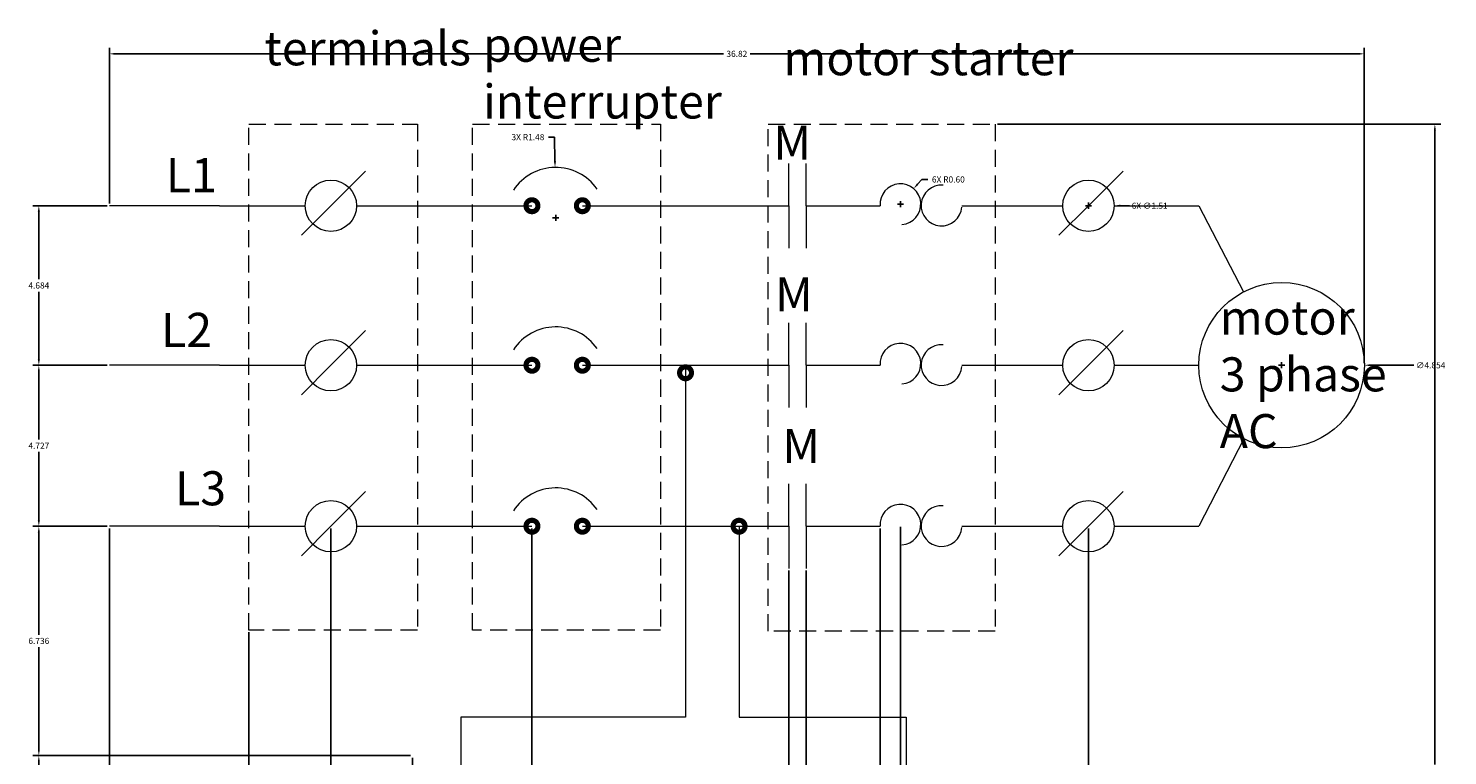
# Model space of a CAD drawing. Units: millimetres. Extents: x 39.4 to 81, y 9.5 to 52.5.
# Tile 2 of 2: x 39.4 to 81, y 31.2 to 52.5. Entities that reach past the tile are written whole.
import ezdxf

# ---------------------------------------------------------------- set-up
doc = ezdxf.new("R2010")
doc.units = ezdxf.units.MM
doc.header["$MEASUREMENT"] = 0
doc.linetypes.add('HIDDENX2', pattern=[0.75, 0.5, -0.25])
for name, color, linetype, lineweight in [('A-ANNO-DIMS', 2, 'Continuous', 18), ('E-ANNO-TEXT', 7, 'Continuous', 13), ('E-DIAG-CONN', 7, 'Continuous', 18), ('E-DIAG-PROT', 7, 'Continuous', 18), ('E-EQPM-BNDY', 8, 'HIDDENX2', 13), ('E-POWR-EQPM', 7, 'Continuous', 20), ('E-POWR-WIRE', 7, 'Continuous', 18)]:
    doc.layers.add(name, color=color, linetype=linetype, lineweight=lineweight)
doc.styles.get("Standard").update_dxf_attribs({"font": 'arial.ttf'})
doc.dimstyles.get("Standard").update_dxf_attribs({"dimtxt": 0.18, "dimasz": 0.18, "dimexe": 0.18, "dimexo": 0.0625, "dimgap": 0.09, "dimtad": 0, "dimtih": 1, "dimtoh": 1, "dimdec": 4, "dimzin": 0, "dimdsep": 46, "dimtxsty": 'Standard', "dimcen": 0.09, "dimadec": 0, "dimazin": 0, "dimtfac": 1, "dimtdec": 4, "dimtofl": 0, "dimtmove": 0, "dimatfit": 3, "dimfxl": 1, "dimtolj": 1, "dimtzin": 0, "dimarcsym": 0})

# ---------------------------------------------------------------- blocks, each defined once
blk = doc.blocks.new('SCREW-TERMINAL')
for q in [(1.883, 1.883), (0, 0)]:
    blk.add_line((0.865, 0.865), q)
blk.add_circle((0.865, 0.865), 0.753)
blk = doc.blocks.new('INTERRUPTER-POLE')
at = {"const_width": 0.15}
for points in [[(0.367, 0.175, 1), (0.717, 0.175, 1)], [(1.846, 0.175, 1), (2.196, 0.175, 1)]]:
    blk.add_lwpolyline(points, format="xyb", close=True, dxfattribs=at)
blk.add_arc((1.239, -0.182), 1.482, 34.8147, 146.7068)
blk = doc.blocks.new('CONTACTOR-NO-POLE')
for p, q in [((0, 1.242), (0, 2.485)), ((0.513, 1.242), (0.513, 2.485)), ((0, 1.242), (0, 0)), ((0.513, 1.242), (0.513, 0))]:
    blk.add_line(p, q)
blk = doc.blocks.new('OVERLOAD-HEATER')
for centre, start, end in [((0.597, 0.638), 274.3585, 184.3585), ((1.802, 0.598), 85.6415, 355.6415)]:
    blk.add_arc(centre, 0.598, start, end)
blk = doc.blocks.new('WIRE-JUNCTION')
at = {"const_width": 0.15}
blk.add_lwpolyline([(0, 0.175, 1), (0.35, 0.175, 1)], format="xyb", close=True, dxfattribs=at)
blk = doc.blocks.new('*D6')
at = {"layer": 'A-ANNO-DIMS', "color": 0, "lineweight": -2, "transparency": 16777216}
for p, q in [((41.706, 47.307), (39.52, 47.307)), ((39.7, 47.127), (39.7, 45.147)), ((39.7, 42.803), (39.7, 44.783)), ((41.706, 42.623), (39.52, 42.623))]:
    blk.add_line(p, q, dxfattribs=at)
at = {"layer": 'A-ANNO-DIMS', "color": 0, "transparency": 16777216}
for points in [[(39.67, 47.127), (39.73, 47.127), (39.7, 47.307)], [(39.67, 42.803), (39.73, 42.803), (39.7, 42.623)]]:
    blk.add_solid(points, dxfattribs=at)
at = {"layer": 'Defpoints', "color": 0, "transparency": 16777216}
for p in [(41.769, 47.307), (39.7, 42.623), (41.769, 42.623)]:
    blk.add_point(p, dxfattribs=at)
at = {"layer": 'A-ANNO-DIMS', "color": 0, "transparency": 16777216, "insert": (39.7, 44.965), "char_height": 0.18, "attachment_point": 5}
blk.add_mtext('\\A1;4.684', dxfattribs=at)
blk = doc.blocks.new('*D7')
at = {"layer": 'A-ANNO-DIMS', "color": 0, "lineweight": -2, "transparency": 16777216}
for p, q in [((41.706, 42.623), (39.52, 42.623)), ((39.7, 42.443), (39.7, 40.44)), ((39.7, 38.076), (39.7, 40.079)), ((41.706, 37.896), (39.52, 37.896))]:
    blk.add_line(p, q, dxfattribs=at)
at = {"layer": 'A-ANNO-DIMS', "color": 0, "transparency": 16777216}
for points in [[(39.67, 42.443), (39.73, 42.443), (39.7, 42.623)], [(39.67, 38.076), (39.73, 38.076), (39.7, 37.896)]]:
    blk.add_solid(points, dxfattribs=at)
at = {"layer": 'Defpoints', "color": 0, "transparency": 16777216}
for p in [(41.769, 42.623), (39.7, 37.896), (41.769, 37.896)]:
    blk.add_point(p, dxfattribs=at)
at = {"layer": 'A-ANNO-DIMS', "color": 0, "transparency": 16777216, "insert": (39.7, 40.26), "char_height": 0.18, "attachment_point": 5}
blk.add_mtext('\\A1;4.727', dxfattribs=at)
blk = doc.blocks.new('*D8')
at = {"layer": 'A-ANNO-DIMS', "color": 0, "lineweight": -2, "transparency": 16777216}
for p, q in [((41.706, 37.896), (39.52, 37.896)), ((39.7, 37.716), (39.7, 34.71)), ((39.7, 31.339), (39.7, 34.346)), ((50.604, 31.159), (39.52, 31.159))]:
    blk.add_line(p, q, dxfattribs=at)
at = {"layer": 'A-ANNO-DIMS', "color": 0, "transparency": 16777216}
for points in [[(39.67, 37.716), (39.73, 37.716), (39.7, 37.896)], [(39.67, 31.339), (39.73, 31.339), (39.7, 31.159)]]:
    blk.add_solid(points, dxfattribs=at)
at = {"layer": 'Defpoints', "color": 0, "transparency": 16777216}
for p in [(41.769, 37.896), (39.7, 31.159), (50.667, 31.159)]:
    blk.add_point(p, dxfattribs=at)
at = {"layer": 'A-ANNO-DIMS', "color": 0, "transparency": 16777216, "insert": (39.7, 34.528), "char_height": 0.18, "attachment_point": 5}
blk.add_mtext('\\A1;6.736', dxfattribs=at)
blk = doc.blocks.new('*D9')
at = {"layer": 'A-ANNO-DIMS', "color": 0, "lineweight": -2, "transparency": 16777216}
for p, q in [((50.604, 31.159), (39.52, 31.159)), ((39.7, 30.979), (39.7, 28.521)), ((39.7, 25.698), (39.7, 28.157)), ((49.021, 25.518), (39.52, 25.518))]:
    blk.add_line(p, q, dxfattribs=at)
at = {"layer": 'A-ANNO-DIMS', "color": 0, "transparency": 16777216}
for points in [[(39.67, 30.979), (39.73, 30.979), (39.7, 31.159)], [(39.67, 25.698), (39.73, 25.698), (39.7, 25.518)]]:
    blk.add_solid(points, dxfattribs=at)
at = {"layer": 'Defpoints', "color": 0, "transparency": 16777216}
for p in [(50.667, 31.159), (39.7, 25.518), (49.084, 25.518)]:
    blk.add_point(p, dxfattribs=at)
at = {"layer": 'A-ANNO-DIMS', "color": 0, "transparency": 16777216, "insert": (39.7, 28.339), "char_height": 0.18, "attachment_point": 5}
blk.add_mtext('\\A1;5.641', dxfattribs=at)
blk = doc.blocks.new('*D12')
at = {"layer": 'A-ANNO-DIMS', "color": 0, "lineweight": -2, "transparency": 16777216}
for p, q in [((41.769, 37.833), (41.769, 9.486)), ((48.27, 37.833), (48.27, 9.486)), ((41.949, 9.666), (44.643, 9.666)), ((48.09, 9.666), (45.396, 9.666))]:
    blk.add_line(p, q, dxfattribs=at)
at = {"layer": 'A-ANNO-DIMS', "color": 0, "transparency": 16777216}
for points in [[(41.949, 9.696), (41.949, 9.636), (41.769, 9.666)], [(48.09, 9.696), (48.09, 9.636), (48.27, 9.666)]]:
    blk.add_solid(points, dxfattribs=at)
at = {"layer": 'Defpoints', "color": 0, "transparency": 16777216}
for p in [(41.769, 37.896), (48.27, 37.896), (48.27, 9.666)]:
    blk.add_point(p, dxfattribs=at)
at = {"layer": 'A-ANNO-DIMS', "color": 0, "transparency": 16777216, "insert": (45.02, 9.666), "char_height": 0.18, "attachment_point": 5}
blk.add_mtext('\\A1;6.501', dxfattribs=at)
blk = doc.blocks.new('*D13')
at = {"layer": 'A-ANNO-DIMS', "color": 0, "lineweight": -2, "transparency": 16777216}
for p, q in [((48.27, 37.833), (48.27, 9.486)), ((54.169, 37.833), (54.169, 9.486)), ((48.45, 9.666), (50.826, 9.666)), ((53.989, 9.666), (51.614, 9.666))]:
    blk.add_line(p, q, dxfattribs=at)
at = {"layer": 'A-ANNO-DIMS', "color": 0, "transparency": 16777216}
for points in [[(48.45, 9.696), (48.45, 9.636), (48.27, 9.666)], [(53.989, 9.696), (53.989, 9.636), (54.169, 9.666)]]:
    blk.add_solid(points, dxfattribs=at)
at = {"layer": 'Defpoints', "color": 0, "transparency": 16777216}
for p in [(48.27, 37.896), (54.169, 37.896), (54.169, 9.666)]:
    blk.add_point(p, dxfattribs=at)
at = {"layer": 'A-ANNO-DIMS', "color": 0, "transparency": 16777216, "insert": (51.22, 9.666), "char_height": 0.18, "attachment_point": 5}
blk.add_mtext('\\A1;5.899', dxfattribs=at)
blk = doc.blocks.new('*D14')
at = {"layer": 'A-ANNO-DIMS', "color": 0, "lineweight": -2, "transparency": 16777216}
for p, q in [((54.169, 37.833), (54.169, 9.486)), ((61.702, 36.591), (61.702, 9.486)), ((54.349, 9.666), (57.543, 9.666)), ((61.522, 9.666), (58.329, 9.666))]:
    blk.add_line(p, q, dxfattribs=at)
at = {"layer": 'A-ANNO-DIMS', "color": 0, "transparency": 16777216}
for points in [[(54.349, 9.696), (54.349, 9.636), (54.169, 9.666)], [(61.522, 9.696), (61.522, 9.636), (61.702, 9.666)]]:
    blk.add_solid(points, dxfattribs=at)
at = {"layer": 'Defpoints', "color": 0, "transparency": 16777216}
for p in [(54.169, 37.896), (61.702, 36.653), (61.702, 9.666)]:
    blk.add_point(p, dxfattribs=at)
at = {"layer": 'A-ANNO-DIMS', "color": 0, "transparency": 16777216, "insert": (57.936, 9.666), "char_height": 0.18, "attachment_point": 5}
blk.add_mtext('\\A1;7.533', dxfattribs=at)
blk = doc.blocks.new('*D15')
at = {"layer": 'A-ANNO-DIMS', "color": 0, "lineweight": -2, "transparency": 16777216}
for p, q in [((64.384, 37.833), (64.384, 9.486)), ((62.215, 36.591), (62.215, 9.486)), ((62.395, 9.666), (62.904, 9.666)), ((64.204, 9.666), (63.695, 9.666))]:
    blk.add_line(p, q, dxfattribs=at)
at = {"layer": 'A-ANNO-DIMS', "color": 0, "transparency": 16777216}
for points in [[(62.395, 9.696), (62.395, 9.636), (62.215, 9.666)], [(64.204, 9.696), (64.204, 9.636), (64.384, 9.666)]]:
    blk.add_solid(points, dxfattribs=at)
at = {"layer": 'Defpoints', "color": 0, "transparency": 16777216}
for p in [(64.384, 37.896), (62.215, 36.653), (64.384, 9.666)]:
    blk.add_point(p, dxfattribs=at)
at = {"layer": 'A-ANNO-DIMS', "color": 0, "transparency": 16777216, "insert": (63.3, 9.666), "char_height": 0.18, "attachment_point": 5}
blk.add_mtext('\\A1;2.169', dxfattribs=at)
blk = doc.blocks.new('*D16')
at = {"layer": 'A-ANNO-DIMS', "color": 0, "lineweight": -2, "transparency": 16777216}
for p, q in [((64.98, 37.879), (64.98, 9.486)), ((70.498, 37.833), (70.498, 9.486)), ((65.16, 9.666), (67.345, 9.666)), ((70.318, 9.666), (68.133, 9.666))]:
    blk.add_line(p, q, dxfattribs=at)
at = {"layer": 'A-ANNO-DIMS', "color": 0, "transparency": 16777216}
for points in [[(65.16, 9.696), (65.16, 9.636), (64.98, 9.666)], [(70.318, 9.696), (70.318, 9.636), (70.498, 9.666)]]:
    blk.add_solid(points, dxfattribs=at)
at = {"layer": 'Defpoints', "color": 0, "transparency": 16777216}
for p in [(64.98, 37.941), (70.498, 37.896), (70.498, 9.666)]:
    blk.add_point(p, dxfattribs=at)
at = {"layer": 'A-ANNO-DIMS', "color": 0, "transparency": 16777216, "insert": (67.739, 9.666), "char_height": 0.18, "attachment_point": 5}
blk.add_mtext('\\A1;5.517', dxfattribs=at)
blk = doc.blocks.new('*D21')
at = {"layer": 'A-ANNO-DIMS', "color": 0, "lineweight": -2, "transparency": 16777216}
for p, q in [((41.769, 47.37), (41.769, 51.948)), ((41.949, 51.768), (59.788, 51.768)), ((78.412, 51.768), (60.573, 51.768)), ((78.592, 42.686), (78.592, 51.948))]:
    blk.add_line(p, q, dxfattribs=at)
at = {"layer": 'A-ANNO-DIMS', "color": 0, "transparency": 16777216}
for points in [[(41.949, 51.798), (41.949, 51.738), (41.769, 51.768)], [(78.412, 51.798), (78.412, 51.738), (78.592, 51.768)]]:
    blk.add_solid(points, dxfattribs=at)
at = {"layer": 'Defpoints', "color": 0, "transparency": 16777216}
for p in [(78.592, 51.768), (41.769, 47.307), (78.592, 42.623)]:
    blk.add_point(p, dxfattribs=at)
at = {"layer": 'A-ANNO-DIMS', "color": 0, "transparency": 16777216, "insert": (60.181, 51.768), "char_height": 0.18, "attachment_point": 5}
blk.add_mtext('\\A1;36.82', dxfattribs=at)
blk = doc.blocks.new('*D22')
at = {"layer": 'A-ANNO-DIMS', "color": 0, "lineweight": -2, "transparency": 16777216}
for p, q in [((67.825, 49.7), (80.841, 49.7)), ((80.661, 49.52), (80.661, 30.899)), ((80.661, 11.915), (80.661, 30.535)), ((49.139, 11.735), (80.841, 11.735))]:
    blk.add_line(p, q, dxfattribs=at)
at = {"layer": 'A-ANNO-DIMS', "color": 0, "transparency": 16777216}
for points in [[(80.631, 49.52), (80.691, 49.52), (80.661, 49.7)], [(80.631, 11.915), (80.691, 11.915), (80.661, 11.735)]]:
    blk.add_solid(points, dxfattribs=at)
at = {"layer": 'Defpoints', "color": 0, "transparency": 16777216}
for p in [(67.763, 49.7), (49.077, 11.735), (80.661, 11.735)]:
    blk.add_point(p, dxfattribs=at)
at = {"layer": 'A-ANNO-DIMS', "color": 0, "transparency": 16777216, "insert": (80.661, 30.717), "char_height": 0.18, "attachment_point": 5}
blk.add_mtext('\\A1;37.965', dxfattribs=at)
blk = doc.blocks.new('*D23')
at = {"layer": 'A-ANNO-DIMS', "color": 0, "lineweight": -2, "transparency": 16777216}
for p, q in [((45.864, 34.781), (45.864, 9.486)), ((50.667, 31.097), (50.667, 9.486)), ((46.044, 9.666), (47.868, 9.666)), ((50.487, 9.666), (48.663, 9.666))]:
    blk.add_line(p, q, dxfattribs=at)
at = {"layer": 'A-ANNO-DIMS', "color": 0, "transparency": 16777216}
for points in [[(46.044, 9.696), (46.044, 9.636), (45.864, 9.666)], [(50.487, 9.696), (50.487, 9.636), (50.667, 9.666)]]:
    blk.add_solid(points, dxfattribs=at)
at = {"layer": 'Defpoints', "color": 0, "transparency": 16777216}
for p in [(45.864, 34.843), (50.667, 31.159), (50.667, 9.666)]:
    blk.add_point(p, dxfattribs=at)
at = {"layer": 'A-ANNO-DIMS', "color": 0, "transparency": 16777216, "insert": (48.265, 9.666), "char_height": 0.18, "attachment_point": 5}
blk.add_mtext('\\A1;4.803', dxfattribs=at)
blk = doc.blocks.new('*D24')
at = {"layer": 'A-ANNO-DIMS', "color": 0, "lineweight": -2, "transparency": 16777216}
for p, q in [((76.075, 42.623), (76.255, 42.623)), ((76.165, 42.533), (76.165, 42.713)), ((80.049, 42.623), (78.772, 42.623))]:
    blk.add_line(p, q, dxfattribs=at)
at = {"layer": 'A-ANNO-DIMS', "color": 0, "transparency": 16777216}
blk.add_solid([(78.772, 42.653), (78.772, 42.593), (78.592, 42.623)], dxfattribs=at)
at = {"layer": 'Defpoints', "color": 0, "transparency": 16777216}
for p in [(73.738, 42.624), (78.592, 42.623)]:
    blk.add_point(p, dxfattribs=at)
at = {"layer": 'A-ANNO-DIMS', "color": 0, "transparency": 16777216, "insert": (80.54, 42.623), "char_height": 0.18, "attachment_point": 5}
blk.add_mtext('\\A1;∅4.854', dxfattribs=at)
blk = doc.blocks.new('*D26')
at = {"layer": 'A-ANNO-DIMS', "color": 0, "lineweight": -2, "transparency": 16777216}
for p, q in [((54.654, 49.321), (54.834, 49.321)), ((54.834, 49.321), (54.844, 48.612)), ((54.776, 46.949), (54.956, 46.949)), ((54.866, 46.859), (54.866, 47.039))]:
    blk.add_line(p, q, dxfattribs=at)
at = {"layer": 'A-ANNO-DIMS', "color": 0, "transparency": 16777216}
blk.add_solid([(54.874, 48.612), (54.814, 48.611), (54.846, 48.432)], dxfattribs=at)
at = {"layer": 'Defpoints', "color": 0, "transparency": 16777216}
for p in [(54.846, 48.432), (54.866, 46.949)]:
    blk.add_point(p, dxfattribs=at)
at = {"layer": 'A-ANNO-DIMS', "color": 0, "transparency": 16777216, "insert": (54.051, 49.321), "char_height": 0.18, "attachment_point": 5}
blk.add_mtext('\\A1;3X R1.48', dxfattribs=at)
blk = doc.blocks.new('*D28')
at = {"layer": 'A-ANNO-DIMS', "color": 0, "lineweight": -2, "transparency": 16777216}
for p, q in [((70.408, 47.307), (70.588, 47.307)), ((70.498, 47.217), (70.498, 47.397)), ((71.702, 47.307), (71.43, 47.307))]:
    blk.add_line(p, q, dxfattribs=at)
at = {"layer": 'A-ANNO-DIMS', "color": 0, "transparency": 16777216}
blk.add_solid([(71.43, 47.337), (71.43, 47.277), (71.25, 47.307)], dxfattribs=at)
at = {"layer": 'Defpoints', "color": 0, "transparency": 16777216}
for p in [(69.745, 47.307), (71.25, 47.307)]:
    blk.add_point(p, dxfattribs=at)
at = {"layer": 'A-ANNO-DIMS', "color": 0, "transparency": 16777216, "insert": (72.295, 47.307), "char_height": 0.18, "attachment_point": 5}
blk.add_mtext('\\A1;6X ∅1.51', dxfattribs=at)
blk = doc.blocks.new('*D29')
at = {"layer": 'A-ANNO-DIMS', "color": 0, "lineweight": -2, "transparency": 16777216}
for p, q in [((65.604, 48.079), (65.486, 47.943)), ((65.784, 48.079), (65.604, 48.079)), ((64.89, 47.353), (65.07, 47.353)), ((64.98, 47.263), (64.98, 47.443))]:
    blk.add_line(p, q, dxfattribs=at)
at = {"layer": 'A-ANNO-DIMS', "color": 0, "transparency": 16777216}
blk.add_solid([(65.464, 47.962), (65.509, 47.923), (65.369, 47.806)], dxfattribs=at)
at = {"layer": 'Defpoints', "color": 0, "transparency": 16777216}
for p in [(65.369, 47.806), (64.98, 47.353)]:
    blk.add_point(p, dxfattribs=at)
at = {"layer": 'A-ANNO-DIMS', "color": 0, "transparency": 16777216, "insert": (66.387, 48.079), "char_height": 0.18, "attachment_point": 5}
blk.add_mtext('\\A1;6X R0.60', dxfattribs=at)

msp = doc.modelspace()

# ---------------------------------------------------------------- linework, layer by layer
at = {"layer": 'E-EQPM-BNDY'}
for points in [[(45.8641, 49.6995), (50.809, 49.6995), (50.809, 34.8433), (45.8641, 34.8433)], [(52.4236, 49.6995), (57.9404, 49.6995), (57.9404, 34.8433), (52.4236, 34.8433)], [(61.1025, 49.6995), (67.763, 49.6995), (67.763, 34.8097), (61.1025, 34.8097)]]:
    msp.add_lwpolyline(points, close=True, dxfattribs=at)
at = {"layer": 'E-POWR-EQPM'}
msp.add_circle((76.1651, 42.6234), 2.4272, dxfattribs=at)
at = {"layer": 'E-POWR-WIRE'}
for p, q in [((44.9971, 47.3072), (41.7689, 47.3072)), ((44.9971, 47.3072), (47.5173, 47.3072)), ((49.023, 47.3072), (54.1694, 47.3072)), ((55.6484, 47.3072), (61.7024, 47.3072)), ((62.2151, 47.3072), (64.3842, 47.3072)), ((66.7827, 47.3072), (69.7447, 47.3072)), ((71.2504, 47.3072), (73.7379, 47.3072)), ((73.7379, 47.3072), (75.0484, 44.7784)), ((44.9971, 42.6234), (41.7689, 42.6234)), ((44.9971, 42.6234), (47.5173, 42.6234)), ((49.023, 42.6234), (54.1694, 42.6234)), ((55.6484, 42.6234), (61.7024, 42.6234)), ((58.6754, 42.6234), (58.6754, 32.2872)), ((62.2151, 42.6234), (64.3842, 42.6234)), ((66.7827, 42.6234), (69.7447, 42.6234)), ((71.2504, 42.6234), (73.7379, 42.6234)), ((75.0565, 40.4641), (73.7379, 37.8959)), ((44.9971, 37.8959), (41.7689, 37.8959)), ((44.9971, 37.8959), (47.5173, 37.8959)), ((49.023, 37.8959), (54.1694, 37.8959)), ((55.6484, 37.8959), (61.7024, 37.8959)), ((60.246, 37.8959), (60.246, 32.2872)), ((62.2151, 37.8959), (64.3842, 37.8959)), ((66.7827, 37.8959), (69.7447, 37.8959)), ((71.2504, 37.8959), (73.7379, 37.8959)), ((58.6754, 32.2872), (52.0845, 32.2872)), ((52.0845, 32.2872), (52.0845, 30.0317)), ((60.246, 32.2872), (65.1455, 32.2872)), ((65.1455, 32.2872), (65.1455, 30.0317))]:
    msp.add_line(p, q, dxfattribs=at)

# ---------------------------------------------------------------- block references
at = {"layer": 'E-DIAG-CONN'}
for name, p in [('SCREW-TERMINAL', (47.405, 46.4419)), ('SCREW-TERMINAL', (69.6323, 46.4419)), ('SCREW-TERMINAL', (47.405, 41.758)), ('SCREW-TERMINAL', (69.6323, 41.758)), ('WIRE-JUNCTION', (58.5002, 42.2264)), ('SCREW-TERMINAL', (47.405, 37.0305)), ('SCREW-TERMINAL', (69.6323, 37.0305)), ('WIRE-JUNCTION', (60.0708, 37.7205))]:
    msp.add_blockref(name, p, dxfattribs=at)
at = {"layer": 'E-DIAG-PROT'}
for name, p in [('INTERRUPTER-POLE', (53.627, 47.1319)), ('OVERLOAD-HEATER', (64.383, 46.7149)), ('INTERRUPTER-POLE', (53.627, 42.448)), ('OVERLOAD-HEATER', (64.383, 42.031)), ('INTERRUPTER-POLE', (53.627, 37.7205)), ('OVERLOAD-HEATER', (64.383, 37.3035))]:
    msp.add_blockref(name, p, dxfattribs=at)
at = {"layer": 'E-POWR-EQPM'}
for p in [(61.702, 46.0649), (61.702, 41.381), (61.702, 36.6535)]:
    msp.add_blockref('CONTACTOR-NO-POLE', p, dxfattribs=at)

# ---------------------------------------------------------------- texts
at = {"layer": 'E-ANNO-TEXT', "char_height": 1, "attachment_point": 1}
for s, width, insert in [('terminals', 2.308794, (46.3155, 52.4292)), ('power interrupter', 2.308794, (52.7312, 52.5344)), ('motor starter', 8.561895, (61.5433, 52.1382)), ('M', 2.308794, (61.2506, 49.6577)), ('L1', 2.308794, (43.426, 48.7039)), ('M', 2.308794, (61.3026, 45.2048)), ('L2', 2.308794, (43.2835, 44.1615)), ('motor\\P3 phase\\PAC', 6.782816, (74.3486, 44.5226)), ('M', 2.308794, (61.5152, 40.7548)), ('L3', 2.308794, (43.6966, 39.5105))]:
    msp.add_mtext_dynamic_manual_height_columns(s, width=width, gutter_width=1, heights=[0], dxfattribs=dict(at, insert=insert))

# ---------------------------------------------------------------- dimensions: what is measured, and where the dimension line sits
at = {"layer": 'A-ANNO-DIMS'}
for base, p1, p2, override, picture, middle in [((78.5924, 51.768), (41.7689, 47.3072), (78.5924, 42.6234), {"dimdec": 2, "dimlfac": 1, "dimrnd": 0, "dimzin": 0, "dimdsep": 46, "dimlunit": 2}, '*D21', (60.1806, 51.768)), ((48.2702, 9.6662), (41.7689, 37.8959), (48.2702, 37.8959), {"dimdec": 3, "dimlfac": 1, "dimrnd": 0, "dimzin": 0, "dimdsep": 46, "dimlunit": 2}, '*D12', (45.0195, 9.6662)), ((54.1694, 9.6662), (48.2702, 37.8959), (54.1694, 37.8959), {"dimdec": 3, "dimlfac": 1, "dimrnd": 0, "dimzin": 0, "dimdsep": 46, "dimlunit": 2}, '*D13', (51.2198, 9.6662)), ((61.7024, 9.6662), (54.1694, 37.8959), (61.7024, 36.6533), {"dimdec": 3, "dimlfac": 1, "dimrnd": 0, "dimzin": 0, "dimdsep": 46, "dimlunit": 2}, '*D14', (57.9359, 9.6662)), ((64.3842, 9.6662), (62.2151, 36.6533), (64.3842, 37.8959), {"dimdec": 3, "dimlfac": 1, "dimrnd": 0, "dimzin": 0, "dimdsep": 46, "dimlunit": 2}, '*D15', (63.2997, 9.6662)), ((70.4975, 9.6662), (64.9801, 37.9414), (70.4975, 37.8959), {"dimdec": 3, "dimlfac": 1, "dimrnd": 0, "dimzin": 0, "dimdsep": 46, "dimlunit": 2}, '*D16', (67.7388, 9.6662)), ((50.6667, 9.6662), (45.8641, 34.8433), (50.6667, 31.1595), {"dimdec": 3, "dimlfac": 1, "dimrnd": 0, "dimzin": 0, "dimdsep": 46, "dimlunit": 2}, '*D23', (48.2654, 9.6662))]:
    dim = msp.add_linear_dim(base=base, p1=p1, p2=p2, dimstyle='Standard', override=override, dxfattribs=at)
    dim.commit()
    dim.dimension.update_dxf_attribs({"geometry": picture, "text_midpoint": middle})
for base, p1, p2, picture, middle in [((80.6609, 11.7347), (67.763, 49.6995), (49.0765, 11.7347), '*D22', (80.6609, 30.7171)), ((39.7004, 42.6234), (41.7689, 47.3072), (41.7689, 42.6234), '*D6', (39.7004, 44.9653)), ((39.70039, 37.89594), (41.76889, 42.62339), (41.76889, 37.89594), '*D7', (39.70039, 40.25967)), ((39.7004, 31.1595), (41.7689, 37.8959), (50.6667, 31.1595), '*D8', (39.7004, 34.5277)), ((39.7004, 25.5184), (50.6667, 31.1595), (49.0837, 25.5184), '*D9', (39.7004, 28.339))]:
    dim = msp.add_linear_dim(base=base, p1=p1, p2=p2, angle=90, dimstyle='Standard', override={"dimdec": 3, "dimlfac": 1, "dimrnd": 0, "dimzin": 0, "dimdsep": 46, "dimlunit": 2}, dxfattribs=at)
    dim.commit()
    dim.dimension.update_dxf_attribs({"geometry": picture, "text_midpoint": middle})
dim = msp.add_radius_dim(center=(54.8657, 46.9494), mpoint=(54.846, 48.4316), text='3X <>', dimstyle='Standard', override={"dimdec": 2, "dimlfac": 1, "dimrnd": 0, "dimzin": 0, "dimdsep": 46, "dimlunit": 2}, dxfattribs=at)
dim.commit()
dim.dimension.update_dxf_attribs({"geometry": '*D26', "text_midpoint": (54.0508, 49.3208), "dimtype": 164})
dim = msp.add_radius_dim(center=(64.9801, 47.3527), mpoint=(65.3692, 47.8062), text='6X <>', dimstyle='Standard', override={"dimdec": 2, "dimlfac": 1, "dimrnd": 0, "dimzin": 0, "dimdsep": 46, "dimlunit": 2}, dxfattribs=at)
dim.commit()
dim.dimension.update_dxf_attribs({"geometry": '*D29', "text_midpoint": (66.3871, 48.0795)})
dim = msp.add_diameter_dim_2p(p1=(69.7447, 47.3075), p2=(71.2504, 47.307), text='6X <>', dimstyle='Standard', override={"dimdec": 2, "dimlfac": 1, "dimrnd": 0, "dimzin": 0, "dimdsep": 46, "dimlunit": 2}, dxfattribs=at)
dim.commit()
dim.dimension.update_dxf_attribs({"geometry": '*D28', "text_midpoint": (71.7021, 47.3069), "dimtype": 163})
dim = msp.add_diameter_dim_2p(p1=(73.73791, 42.62379), p2=(78.59236, 42.623), dimstyle='Standard', override={"dimdec": 3, "dimlfac": 1, "dimrnd": 0, "dimzin": 0, "dimdsep": 46, "dimlunit": 2}, dxfattribs=at)
dim.commit()
dim.dimension.update_dxf_attribs({"geometry": '*D24', "text_midpoint": (80.04869, 42.62276), "dimtype": 163})

doc.saveas('drawing.dxf')
